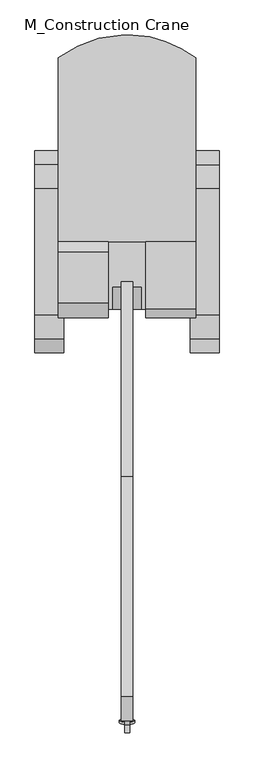
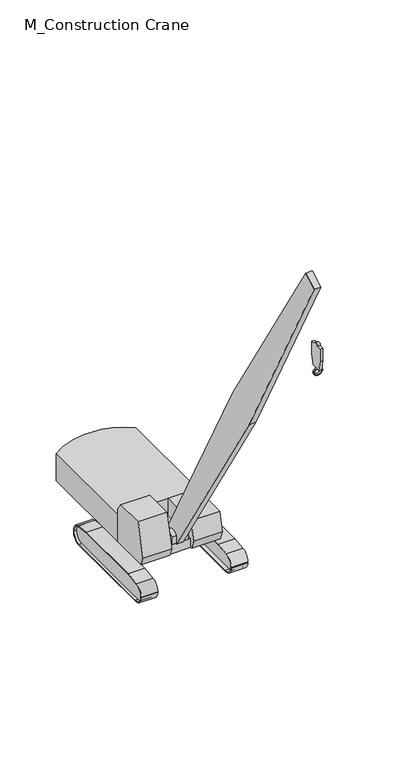
"""IFC4 building model written with IfcOpenShell, lengths in millimetres: geographic element geometry, M_Construction Crane."""

from ifc_helpers import new_model, si_unit, point, frame, frame_2d, origin, place, context, project, spatial, polyline, circle_curve, trimmed, segment, composite_curve, outline, extrude, source, transform, mapped, element, save


def m_construction_crane_c1d51077(model_context):
    return source(origin(), model_context, "Body", "SweptSolid", [
        extrude(outline(composite_curve([segment(polyline([(-651.6384615, 0.0), (-5163.0384615, 0.0)]), True, "CONTINUOUS"), segment(trimmed(circle_curve(frame_2d((-5163.0384615, 431.8)), 431.8), [point((-5163.0384615, 0.0))], [point((-5594.8384615, 431.8))], False, "CARTESIAN"), True, "CONTINUOUS"), segment(polyline([(-5594.8384615, 431.8), (-5594.8384615, 475.1036968)]), True, "CONTINUOUS"), segment(trimmed(circle_curve(frame_2d((-5163.0384615, 475.1036968)), 431.8), [point((-5594.8384615, 475.1036968))], [point((-5217.7268735, 903.4264928))], False, "CARTESIAN"), True, "CONTINUOUS"), segment(polyline([(-5217.7268735, 903.4264928), (-4578.8384615, 985.06875), (-1235.8384615, 985.06875), (-596.9500496, 903.4264928)]), True, "CONTINUOUS"), segment(trimmed(circle_curve(frame_2d((-651.6384615, 475.1036968)), 431.8), [point((-596.9500496, 903.4264928))], [point((-219.8384615, 475.1036968))], False, "CARTESIAN"), True, "CONTINUOUS"), segment(polyline([(-219.8384615, 475.1036968), (-219.8384615, 431.8)]), True, "CONTINUOUS"), segment(trimmed(circle_curve(frame_2d((-651.6384615, 431.8)), 431.8), [point((-219.8384615, 431.8))], [point((-651.6384615, 0.0))], False, "CARTESIAN"), True, "CONTINUOUS")], self_intersect=False), holes=[composite_curve([segment(polyline([(-4575.608491, 934.26875), (-5189.1160735, 855.3847601)]), True, "CONTINUOUS"), segment(trimmed(circle_curve(frame_2d((-5137.6945084, 451.7022639)), 406.9443882), [point((-5189.1160735, 855.3847601))], [point((-5544.6388966, 451.7022639))], True, "CARTESIAN"), True, "CONTINUOUS"), segment(trimmed(circle_curve(frame_2d((-5143.9371049, 451.7022639)), 400.7017917), [point((-5544.6388966, 451.7022639))], [point((-5143.9371049, 51.0004722))], True, "CARTESIAN"), True, "CONTINUOUS"), segment(polyline([(-5143.9371049, 51.0004722), (-676.7161092, 51.0004722)]), True, "CONTINUOUS"), segment(trimmed(circle_curve(frame_2d((-676.7161092, 456.946505)), 405.9460328), [point((-676.7161092, 51.0004722))], [point((-270.7700765, 456.946505))], True, "CARTESIAN"), True, "CONTINUOUS"), segment(trimmed(circle_curve(frame_2d((-676.8331731, 453.2718224)), 406.0797233), [point((-270.7700765, 456.946505))], [point((-625.3121051, 856.0699371))], True, "CARTESIAN"), True, "CONTINUOUS"), segment(polyline([(-625.3121051, 856.0699371), (-1239.0684321, 934.26875), (-4575.608491, 934.26875)]), True, "CONTINUOUS")], self_intersect=False)]), frame((-8129.12123, 0.0, 0.0), z_axis=(1.0, 0.0, 0.0), x_axis=(0.0, 1.0, 0.0)), (0.0, 0.0, 1.0), 762.0),
        extrude(outline(polyline([(-5179.12123, -2642.3288049), (-5179.12123, -4433.7384615), (-6179.12123, -4433.7384615), (-6179.12123, -2642.3288049), (-5179.12123, -2642.3288049)])), frame((0.0, 0.0, 1155.0), z_axis=(0.0, 0.0, 1.0), x_axis=(1.0, 0.0, 0.0)), (0.0, 0.0, 1.0), 434.1377619),
        extrude(outline(composite_curve([segment(polyline([(-3855.5873985, 1944.8065119), (-3855.5873985, 1589.2065119), (-4435.4967838, 1589.2065119), (-4435.4967838, 1944.8065119)]), True, "CONTINUOUS"), segment(trimmed(circle_curve(frame_2d((-4145.5420911, 1746.7297499)), 351.15257), [point((-4435.4967838, 1944.8065119))], [point((-3855.5873985, 1944.8065119))], False, "CARTESIAN"), True, "CONTINUOUS")], self_intersect=False)), frame((-6056.08998, 0.0, 0.0), z_axis=(1.0, 0.0, 0.0), x_axis=(0.0, 1.0, 0.0)), (0.0, 0.0, 1.0), 755.1034902),
        extrude(outline(composite_curve([segment(polyline([(-4575.608491, 934.26875), (-1239.0684321, 934.26875), (-625.3121051, 856.1386871)]), True, "CONTINUOUS"), segment(trimmed(circle_curve(frame_2d((-676.8331731, 453.3411993)), 406.0791014), [point((-625.3121051, 856.1386871))], [point((-270.7700765, 456.946505))], False, "CARTESIAN"), True, "CONTINUOUS"), segment(trimmed(circle_curve(frame_2d((-676.7161092, 456.946505)), 405.9460328), [point((-270.7700765, 456.946505))], [point((-676.7161092, 51.0004722))], False, "CARTESIAN"), True, "CONTINUOUS"), segment(polyline([(-676.7161092, 51.0004722), (-5143.9005487, 51.0004722)]), True, "CONTINUOUS"), segment(trimmed(circle_curve(frame_2d((-5143.9005487, 451.7388201)), 400.738348), [point((-5143.9005487, 51.0004722))], [point((-5544.6388966, 451.7388201))], False, "CARTESIAN"), True, "CONTINUOUS"), segment(trimmed(circle_curve(frame_2d((-5137.6579522, 451.7388201)), 406.9809445), [point((-5544.6388966, 451.7388201))], [point((-5189.1160735, 855.4535101))], False, "CARTESIAN"), True, "CONTINUOUS"), segment(polyline([(-5189.1160735, 855.4535101), (-4575.608491, 934.26875)]), True, "CONTINUOUS")], self_intersect=False)), frame((-8017.4009175, 0.0, 0.0), z_axis=(1.0, 0.0, 0.0), x_axis=(0.0, 1.0, 0.0)), (0.0, 0.0, 1.0), 464.6393791),
        extrude(outline(composite_curve([segment(polyline([(-651.6384615, 0.0), (-5163.0384615, 0.0)]), True, "CONTINUOUS"), segment(trimmed(circle_curve(frame_2d((-5163.0384615, 431.8)), 431.8), [point((-5163.0384615, 0.0))], [point((-5594.8384615, 431.8))], False, "CARTESIAN"), True, "CONTINUOUS"), segment(polyline([(-5594.8384615, 431.8), (-5594.8384615, 475.1036968)]), True, "CONTINUOUS"), segment(trimmed(circle_curve(frame_2d((-5163.0384615, 475.1036968)), 431.8), [point((-5594.8384615, 475.1036968))], [point((-5217.7268735, 903.4264928))], False, "CARTESIAN"), True, "CONTINUOUS"), segment(polyline([(-5217.7268735, 903.4264928), (-4578.8384615, 985.06875), (-1235.8384615, 985.06875), (-596.9500496, 903.4264928)]), True, "CONTINUOUS"), segment(trimmed(circle_curve(frame_2d((-651.6384615, 475.1036968)), 431.8), [point((-596.9500496, 903.4264928))], [point((-219.8384615, 475.1036968))], False, "CARTESIAN"), True, "CONTINUOUS"), segment(polyline([(-219.8384615, 475.1036968), (-219.8384615, 431.8)]), True, "CONTINUOUS"), segment(trimmed(circle_curve(frame_2d((-651.6384615, 431.8)), 431.8), [point((-219.8384615, 431.8))], [point((-651.6384615, 0.0))], False, "CARTESIAN"), True, "CONTINUOUS")], self_intersect=False), holes=[composite_curve([segment(polyline([(-4575.608491, 934.26875), (-5189.1160735, 855.3847601)]), True, "CONTINUOUS"), segment(trimmed(circle_curve(frame_2d((-5137.6945084, 451.7022639)), 406.9443882), [point((-5189.1160735, 855.3847601))], [point((-5544.6388966, 451.7022639))], True, "CARTESIAN"), True, "CONTINUOUS"), segment(trimmed(circle_curve(frame_2d((-5143.9371049, 451.7022639)), 400.7017917), [point((-5544.6388966, 451.7022639))], [point((-5143.9371049, 51.0004722))], True, "CARTESIAN"), True, "CONTINUOUS"), segment(polyline([(-5143.9371049, 51.0004722), (-676.7161092, 51.0004722)]), True, "CONTINUOUS"), segment(trimmed(circle_curve(frame_2d((-676.7161092, 456.946505)), 405.9460328), [point((-676.7161092, 51.0004722))], [point((-270.7700765, 456.946505))], True, "CARTESIAN"), True, "CONTINUOUS"), segment(trimmed(circle_curve(frame_2d((-676.8331731, 453.2718224)), 406.0797233), [point((-270.7700765, 456.946505))], [point((-625.3121051, 856.0699371))], True, "CARTESIAN"), True, "CONTINUOUS"), segment(polyline([(-625.3121051, 856.0699371), (-1239.0684321, 934.26875), (-4575.608491, 934.26875)]), True, "CONTINUOUS")], self_intersect=False)]), frame((-3991.12123, 0.0, 0.0), z_axis=(1.0, 0.0, 0.0), x_axis=(0.0, 1.0, 0.0)), (0.0, 0.0, 1.0), 762.0),
        extrude(outline(composite_curve([segment(polyline([(-4575.608491, 934.26875), (-1239.0684321, 934.26875), (-625.3121051, 856.1386871)]), True, "CONTINUOUS"), segment(trimmed(circle_curve(frame_2d((-676.8331731, 453.3411993)), 406.0791014), [point((-625.3121051, 856.1386871))], [point((-270.7700765, 456.946505))], False, "CARTESIAN"), True, "CONTINUOUS"), segment(trimmed(circle_curve(frame_2d((-676.7161092, 456.946505)), 405.9460328), [point((-270.7700765, 456.946505))], [point((-676.7161092, 51.0004722))], False, "CARTESIAN"), True, "CONTINUOUS"), segment(polyline([(-676.7161092, 51.0004722), (-5143.9371049, 51.0004722)]), True, "CONTINUOUS"), segment(trimmed(circle_curve(frame_2d((-5143.9371049, 451.7022639)), 400.7017917), [point((-5143.9371049, 51.0004722))], [point((-5544.6388966, 451.7022639))], False, "CARTESIAN"), True, "CONTINUOUS"), segment(trimmed(circle_curve(frame_2d((-5137.6945084, 451.7710081)), 406.944394), [point((-5544.6388966, 451.7022639))], [point((-5189.1160735, 855.4535101))], False, "CARTESIAN"), True, "CONTINUOUS"), segment(polyline([(-5189.1160735, 855.4535101), (-4575.608491, 934.26875)]), True, "CONTINUOUS")], self_intersect=False)), frame((-3805.4809216, 0.0, 0.0), z_axis=(1.0, 0.0, 0.0), x_axis=(0.0, 1.0, 0.0)), (0.0, 0.0, 1.0), 464.6393791),
        extrude(outline(polyline([(-2642.3288049, 2759.86875), (-2642.3288049, 2455.06875), (-2642.3288049, 1155.06875), (-4509.1429639, 1155.06875), (-4662.3384615, 1584.1295061), (-4278.9384615, 3110.06875), (-2907.3384615, 3110.06875), (-2642.3288049, 2759.86875)])), frame((-7504.12123, 0.0, 0.0), z_axis=(1.0, 0.0, 0.0), x_axis=(0.0, 1.0, 0.0)), (0.0, 0.0, 1.0), 1325.0),
        extrude(outline(polyline([(-2642.3288049, 1155.06875), (-4509.1429639, 1155.06875), (-4662.3384615, 1584.1295061), (-4443.5105446, 2455.06875), (-2642.3288049, 2455.06875), (-2642.3288049, 1155.06875)])), frame((-5179.12123, 0.0, 0.0), z_axis=(1.0, 0.0, 0.0), x_axis=(0.0, 1.0, 0.0)), (0.0, 0.0, 1.0), 1325.0),
        extrude(outline(composite_curve([segment(polyline([(-7504.12123, -2642.3288049), (-7504.12123, 2248.0711951)]), True, "CONTINUOUS"), segment(trimmed(circle_curve(frame_2d((-5666.4440826, -194.6737798)), 3056.8055728), [point((-7504.12123, 2248.0711951))], [point((-5831.52123, 2857.6711951))], False, "CARTESIAN"), True, "CONTINUOUS"), segment(polyline([(-5831.52123, 2857.6711951), (-5526.72123, 2857.6711951)]), True, "CONTINUOUS"), segment(trimmed(circle_curve(frame_2d((-5627.7327269, -18.8926004)), 2878.3367753), [point((-5526.72123, 2857.6711951))], [point((-3854.12123, 2248.0711951))], False, "CARTESIAN"), True, "CONTINUOUS"), segment(polyline([(-3854.12123, 2248.0711951), (-3854.12123, -2642.3288049), (-7504.12123, -2642.3288049)]), True, "CONTINUOUS")], self_intersect=False)), frame((0.0, 0.0, 1155.0), z_axis=(0.0, 0.0, 1.0), x_axis=(1.0, 0.0, 0.0)), (0.0, 0.0, 1.0), 1300.06875),
        extrude(outline(composite_curve([segment(polyline([(-15283.8512674, 17825.5884876), (-15067.9512674, 17825.5884876), (-15067.9512674, 17215.9884876), (-15156.1645417, 16715.7061491), (-15614.7379931, 16715.7061491), (-15713.9482506, 17215.9884876), (-15713.9482506, 17825.5884876), (-15498.0482506, 17825.5884876)]), True, "CONTINUOUS"), segment(trimmed(circle_curve(frame_2d((-15390.949759, 17825.5884876)), 107.0984916), [point((-15498.0482506, 17825.5884876))], [point((-15283.8512674, 17825.5884876))], False, "CARTESIAN"), True, "CONTINUOUS")], self_intersect=False)), frame((-5743.7360332, 0.0, 0.0), z_axis=(1.0, 0.0, 0.0), x_axis=(0.0, 1.0, 0.0)), (0.0, 0.0, 1.0), 133.1095203),
        extrude(outline(composite_curve([segment(trimmed(circle_curve(frame_2d((0.0, -203.2)), 203.2), [point((0.0, -406.4))], [point((0.0, 0.0))], False, "CARTESIAN"), True, "CONTINUOUS"), segment(trimmed(circle_curve(frame_2d((0.0, -203.2)), 203.2), [point((0.0, 0.0))], [point((0.0, -406.4))], False, "CARTESIAN"), True, "CONTINUOUS")], self_intersect=False), holes=[composite_curve([segment(trimmed(circle_curve(frame_2d((0.0, -203.2)), 152.4), [point((0.0, -355.6))], [point((0.0, -50.8))], True, "CARTESIAN"), True, "CONTINUOUS"), segment(trimmed(circle_curve(frame_2d((0.0, -203.2)), 152.4), [point((0.0, -50.8))], [point((0.0, -355.6))], True, "CARTESIAN"), True, "CONTINUOUS")], self_intersect=False)]), frame((-5475.92123, -15442.2674955, 16542.7514998), z_axis=(0.0, 0.980898446346255, 0.19452053350611384), x_axis=(0.0, -0.19452053350611384, 0.980898446346255)), (0.0, 0.0, 1.0), 62.999),
        extrude(outline(polyline([(-8901.0827225, 11614.0090459), (-3709.0413561, 1909.9296043), (-4412.9468043, 1503.5296043), (-10220.9054378, 10852.0090459), (-15390.949759, 20568.7884876), (-14731.0384013, 20949.7884876), (-8901.0827225, 11614.0090459)])), frame((-5831.52123, 0.0, 0.0), z_axis=(1.0, 0.0, 0.0), x_axis=(0.0, 1.0, 0.0)), (0.0, 0.0, 1.0), 304.8),
    ])


if __name__ == "__main__":
    model = new_model("IFC4")
    model_context = context("Model", 3, world=origin())
    ifc_project = project(units=[si_unit("LENGTHUNIT", "METRE", prefix="MILLI")], contexts=[model_context])
    site = spatial("IfcSite", under=ifc_project)
    building = spatial("IfcBuilding", under=site)
    placement = place(None, origin())
    m_construction_crane_shape = m_construction_crane_c1d51077(model_context)
    element("IfcGeographicElement", 1, ObjectType="M_Construction Crane", at=placement, inside=building, context=model_context, shape_type="MappedRepresentation", body=[
        mapped(m_construction_crane_shape, transform((0.0, 0.0, 0.0), x_axis=(1.0, 0.0, 0.0), y_axis=(0.0, 1.0, 0.0), z_axis=(0.0, 0.0, 1.0))),
    ])
    save(model, "model.ifc")

# Revit data of these elements
# Type "M_Construction Crane"
#   Boom Angle = 60.00°
#   Boom Half = 36' - 1.07087"
#   Boom Length = 72' - 2.14173"
#   Cab Width = 11' - 11.70079"
#   Counter Weight = 18' - 0.53543"
#   Hook = 30.00°
#   Turning Radius = 19' - 0.54333"
#   Width = 16' - 0.91339"
# Element 1 (IfcGeographicElement, "M_Construction Crane")
#   Materials on its faces: "Metal, Paint Finish, White, Matte", "Plastic, Opaque Black", "Steel"
# Materials
#   "Metal, Paint Finish, White, Matte": class "Metal", colour RGB 247 247 239, transparency 0, Description = "Paint finished steel", Cost = 0
#   "Plastic, Opaque Black": class "Plastic", colour RGB 0 0 0, transparency 0.7, Description = "Plastic, generic, opaque black", Cost = 0
#   "Steel": class "Metal", colour RGB 128 128 128, transparency 0, Description = "Steel, mill finish", Cost = 0
